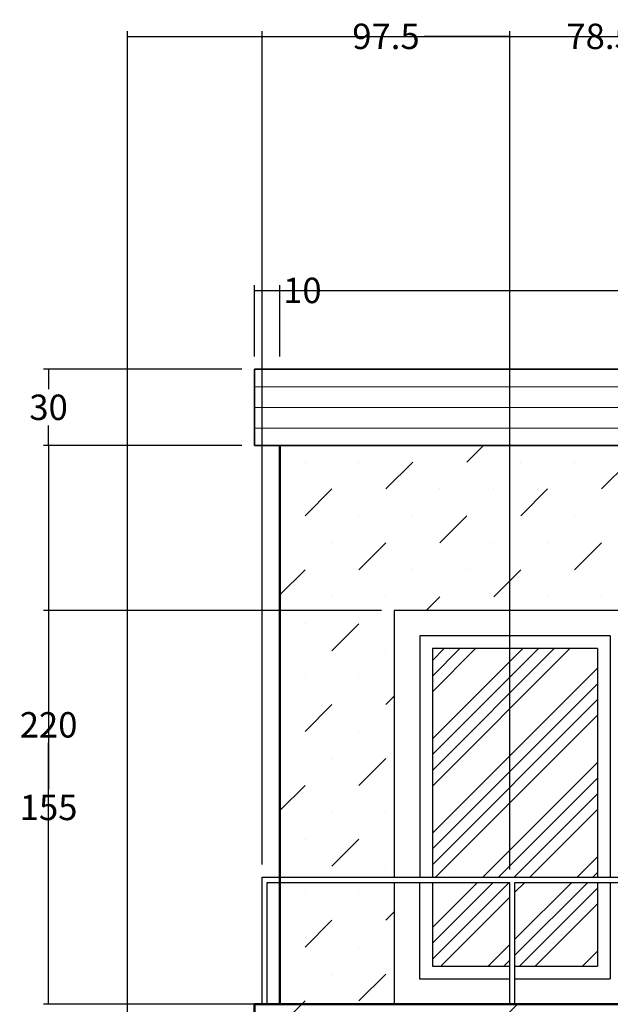
# Model space of a CAD drawing. Units: millimetres. Extents: x 301 to 1039, y -12 to 673.
# Tile 3 of 6: x 301 to 534, y 285 to 673. Entities that reach past the tile are written whole.
import ezdxf

# ---------------------------------------------------------------- set-up
doc = ezdxf.new("R2010")
doc.units = ezdxf.units.MM
doc.header["$MEASUREMENT"] = 0
for name, color, linetype, lineweight in [('A-ANNO-DIMS', 2, 'Continuous', 18), ('A-FLOR-HRAL', 6, 'Continuous', 25), ('A-GLAZ', 4, 'Continuous', 25), ('A-GLAZ-PATT', 8, 'Continuous', 13), ('A-ROOF', 1, 'Continuous', 35), ('A-WALL', 7, 'Continuous', 50), ('A-WALL-PATT', 9, 'Continuous', 13)]:
    doc.layers.add(name, color=color, linetype=linetype, lineweight=lineweight)
doc.styles.get("Standard").update_dxf_attribs({"font": 'arial.ttf'})
doc.dimstyles.get("Standard").update_dxf_attribs({"dimtxt": 10, "dimasz": 0.18, "dimexe": 2, "dimexo": 5, "dimgap": 2, "dimtad": 0, "dimtih": 1, "dimtoh": 1, "dimdec": 0, "dimzin": 0, "dimdsep": 46, "dimtxsty": 'Standard', "dimcen": 0.09, "dimadec": 0, "dimazin": 0, "dimtfac": 1, "dimtdec": 0, "dimtofl": 0, "dimtmove": 0, "dimatfit": 3, "dimfxl": 1, "dimtolj": 1, "dimtzin": 0, "dimarcsym": 0})

# ---------------------------------------------------------------- blocks, each defined once
blk = doc.blocks.new('WIN-SASH-UPPER')
for p, q in [((623.79, 430.09), (548.79, 430.09)), ((548.79, 430.09), (548.79, 400.52)), ((623.79, 430.09), (623.79, 400.52)), ((618.79, 425.09), (553.79, 425.09)), ((553.79, 425.09), (553.79, 400.52)), ((618.79, 425.09), (618.79, 400.52)), ((548.79, 400.52), (548.79, 335.09)), ((553.79, 400.52), (553.79, 335.09)), ((618.79, 400.52), (618.79, 335.09)), ((623.79, 400.52), (623.79, 335.09))]:
    blk.add_line(p, q)
blk = doc.blocks.new('*D20')
at = {"layer": 'A-ANNO-DIMS', "color": 0, "lineweight": -2, "transparency": 16777216}
for p, q in [((343.79, 30.09), (343.79, 668.09)), ((953.79, 30.09), (953.79, 668.09)), ((343.97, 666.09), (635.73, 666.09)), ((953.61, 666.09), (661.85, 666.09))]:
    blk.add_line(p, q, dxfattribs=at)
at = {"layer": 'A-ANNO-DIMS', "color": 0, "transparency": 16777216}
for points in [[(343.97, 666.12), (343.97, 666.06), (343.79, 666.09)], [(953.61, 666.12), (953.61, 666.06), (953.79, 666.09)]]:
    blk.add_solid(points, dxfattribs=at)
at = {"layer": 'Defpoints', "color": 0, "transparency": 16777216}
for p in [(953.79, 666.09), (343.79, 25.09), (953.79, 25.09)]:
    blk.add_point(p, dxfattribs=at)
at = {"layer": 'A-ANNO-DIMS', "color": 0, "transparency": 16777216, "insert": (648.79, 666.09), "char_height": 10, "attachment_point": 5}
blk.add_mtext('\\A1;610', dxfattribs=at)
blk = doc.blocks.new('*D35')
at = {"layer": 'A-ANNO-DIMS', "color": 0, "lineweight": -2, "transparency": 16777216}
for p, q in [((388.79, 505.09), (310.79, 505.09)), ((312.79, 504.91), (312.79, 402.19)), ((312.79, 285.27), (312.79, 387.98)), ((388.79, 285.09), (310.79, 285.09))]:
    blk.add_line(p, q, dxfattribs=at)
at = {"layer": 'A-ANNO-DIMS', "color": 0, "transparency": 16777216}
for points in [[(312.76, 504.91), (312.82, 504.91), (312.79, 505.09)], [(312.76, 285.27), (312.82, 285.27), (312.79, 285.09)]]:
    blk.add_solid(points, dxfattribs=at)
at = {"layer": 'Defpoints', "color": 0, "transparency": 16777216}
for p in [(312.79, 505.09), (393.79, 505.09), (393.79, 285.09)]:
    blk.add_point(p, dxfattribs=at)
at = {"layer": 'A-ANNO-DIMS', "color": 0, "transparency": 16777216, "insert": (312.79, 395.09), "char_height": 10, "attachment_point": 5}
blk.add_mtext('\\A1;220', dxfattribs=at)
blk = doc.blocks.new('*D36')
at = {"layer": 'A-ANNO-DIMS', "color": 0, "lineweight": -2, "transparency": 16777216}
for p, q in [((388.79, 535.09), (310.79, 535.09)), ((312.79, 534.91), (312.79, 527.2)), ((312.79, 505.27), (312.79, 512.98)), ((388.79, 505.09), (310.79, 505.09))]:
    blk.add_line(p, q, dxfattribs=at)
at = {"layer": 'A-ANNO-DIMS', "color": 0, "transparency": 16777216}
for points in [[(312.76, 534.91), (312.82, 534.91), (312.79, 535.09)], [(312.76, 505.27), (312.82, 505.27), (312.79, 505.09)]]:
    blk.add_solid(points, dxfattribs=at)
at = {"layer": 'Defpoints', "color": 0, "transparency": 16777216}
for p in [(312.79, 535.09), (393.79, 535.09), (393.79, 505.09)]:
    blk.add_point(p, dxfattribs=at)
at = {"layer": 'A-ANNO-DIMS', "color": 0, "transparency": 16777216, "insert": (312.79, 520.09), "char_height": 10, "attachment_point": 5}
blk.add_mtext('\\A1;30', dxfattribs=at)
blk = doc.blocks.new('*D43')
at = {"layer": 'A-ANNO-DIMS', "color": 0, "lineweight": -2, "transparency": 16777216}
for p, q in [((393.79, 540.09), (393.79, 568.09)), ((393.97, 566.09), (403.61, 566.09)), ((403.79, 540.09), (403.79, 568.09)), ((403.79, 566.09), (403.97, 566.09))]:
    blk.add_line(p, q, dxfattribs=at)
at = {"layer": 'A-ANNO-DIMS', "color": 0, "transparency": 16777216}
for points in [[(393.97, 566.12), (393.97, 566.06), (393.79, 566.09)], [(403.61, 566.12), (403.61, 566.06), (403.79, 566.09)]]:
    blk.add_solid(points, dxfattribs=at)
at = {"layer": 'Defpoints', "color": 0, "transparency": 16777216}
for p in [(403.79, 566.09), (393.79, 535.09), (403.79, 535.09)]:
    blk.add_point(p, dxfattribs=at)
at = {"layer": 'A-ANNO-DIMS', "color": 0, "transparency": 16777216, "insert": (412.64, 566.09), "char_height": 10, "attachment_point": 5}
blk.add_mtext('\\A1;10', dxfattribs=at)
blk = doc.blocks.new('*D44')
at = {"layer": 'A-ANNO-DIMS', "color": 0, "lineweight": -2, "transparency": 16777216}
for p, q in [((403.79, 540.09), (403.79, 568.09)), ((403.97, 566.09), (540.76, 566.09)), ((703.61, 566.09), (566.82, 566.09)), ((703.79, 540.09), (703.79, 568.09))]:
    blk.add_line(p, q, dxfattribs=at)
at = {"layer": 'A-ANNO-DIMS', "color": 0, "transparency": 16777216}
for points in [[(403.97, 566.12), (403.97, 566.06), (403.79, 566.09)], [(703.61, 566.12), (703.61, 566.06), (703.79, 566.09)]]:
    blk.add_solid(points, dxfattribs=at)
at = {"layer": 'Defpoints', "color": 0, "transparency": 16777216}
for p in [(703.79, 566.09), (403.79, 535.09), (703.79, 535.09)]:
    blk.add_point(p, dxfattribs=at)
at = {"layer": 'A-ANNO-DIMS', "color": 0, "transparency": 16777216, "insert": (553.79, 566.09), "char_height": 10, "attachment_point": 5}
blk.add_mtext('\\A1;300', dxfattribs=at)
blk = doc.blocks.new('*D58')
at = {"layer": 'A-ANNO-DIMS', "color": 0, "lineweight": -2, "transparency": 16777216}
for p, q in [((443.79, 440.09), (310.79, 440.09)), ((312.79, 439.91), (312.79, 369.69)), ((312.79, 285.27), (312.79, 355.48)), ((443.79, 285.09), (310.79, 285.09))]:
    blk.add_line(p, q, dxfattribs=at)
at = {"layer": 'A-ANNO-DIMS', "color": 0, "transparency": 16777216}
for points in [[(312.76, 439.91), (312.82, 439.91), (312.79, 440.09)], [(312.76, 285.27), (312.82, 285.27), (312.79, 285.09)]]:
    blk.add_solid(points, dxfattribs=at)
at = {"layer": 'Defpoints', "color": 0, "transparency": 16777216}
for p in [(312.79, 440.09), (448.79, 440.09), (448.79, 285.09)]:
    blk.add_point(p, dxfattribs=at)
at = {"layer": 'A-ANNO-DIMS', "color": 0, "transparency": 16777216, "insert": (312.79, 362.59), "char_height": 10, "attachment_point": 5}
blk.add_mtext('\\A1;155', dxfattribs=at)
blk = doc.blocks.new('*D59')
at = {"layer": 'A-ANNO-DIMS', "color": 0, "lineweight": -2, "transparency": 16777216}
for p, q in [((396.79, 340.09), (396.79, 668.09)), ((494.29, 338.09), (494.29, 668.09)), ((396.97, 666.09), (430.51, 666.09)), ((494.11, 666.09), (460.56, 666.09))]:
    blk.add_line(p, q, dxfattribs=at)
at = {"layer": 'A-ANNO-DIMS', "color": 0, "transparency": 16777216}
for points in [[(396.97, 666.12), (396.97, 666.06), (396.79, 666.09)], [(494.11, 666.12), (494.11, 666.06), (494.29, 666.09)]]:
    blk.add_solid(points, dxfattribs=at)
at = {"layer": 'Defpoints', "color": 0, "transparency": 16777216}
for p in [(494.29, 666.09), (396.79, 335.09), (494.29, 333.09)]:
    blk.add_point(p, dxfattribs=at)
at = {"layer": 'A-ANNO-DIMS', "color": 0, "transparency": 16777216, "insert": (445.54, 666.09), "char_height": 10, "attachment_point": 5}
blk.add_mtext('\\A1;97.5', dxfattribs=at)
blk = doc.blocks.new('*D60')
at = {"layer": 'A-ANNO-DIMS', "color": 0, "lineweight": -2, "transparency": 16777216}
for p, q in [((494.29, 338.09), (494.29, 668.09)), ((572.8, 338.09), (572.8, 668.09)), ((494.47, 666.09), (515.68, 666.09)), ((572.62, 666.09), (551.41, 666.09))]:
    blk.add_line(p, q, dxfattribs=at)
at = {"layer": 'A-ANNO-DIMS', "color": 0, "transparency": 16777216}
for points in [[(494.47, 666.12), (494.47, 666.06), (494.29, 666.09)], [(572.62, 666.12), (572.62, 666.06), (572.8, 666.09)]]:
    blk.add_solid(points, dxfattribs=at)
at = {"layer": 'Defpoints', "color": 0, "transparency": 16777216}
for p in [(572.8, 666.09), (494.29, 333.09), (572.8, 333.09)]:
    blk.add_point(p, dxfattribs=at)
at = {"layer": 'A-ANNO-DIMS', "color": 0, "transparency": 16777216, "insert": (533.54, 666.09), "char_height": 10, "attachment_point": 5}
blk.add_mtext('\\A1;78.51', dxfattribs=at)

msp = doc.modelspace()

# ---------------------------------------------------------------- hatches: boundary and pattern name
at = {"layer": 'A-GLAZ-PATT'}
h = msp.add_hatch(dxfattribs=at)
h.set_pattern_fill('ANSI34', color=256, scale=35)
h.paths.add_polyline_path([(528.788, 400.52), (528.788, 425.088), (463.788, 425.088), (463.788, 400.52), (463.788, 335.088), (528.788, 335.088)])
h.paths.add_polyline_path([(494.288, 333.088), (463.788, 333.088), (463.788, 300.088), (494.288, 300.088)])
h.paths.add_polyline_path([(528.788, 333.088), (496.288, 333.088), (496.288, 300.088), (528.788, 300.088)])
h.paths.add_polyline_path([(618.788, 400.52), (618.788, 425.088), (553.788, 425.088), (553.788, 400.52), (553.788, 335.088), (618.788, 335.088)])
h.paths.add_polyline_path([(618.788, 333.088), (574.798, 333.088), (574.798, 300.088), (618.788, 300.088)])
h.paths.add_polyline_path([(572.798, 333.088), (553.788, 333.088), (553.788, 300.088), (572.798, 300.088)])
h.paths.add_polyline_path([(501.288, 180.088), (433.788, 180.088), (433.788, 110.088), (501.288, 110.088)])
h.paths.add_polyline_path([(573.788, 180.088), (506.288, 180.088), (506.288, 110.088), (573.788, 110.088)])
h.paths.add_polyline_path([(573.788, 210.088), (506.288, 210.088), (506.288, 185.088), (573.788, 185.088)])
h.paths.add_polyline_path([(501.288, 210.088), (433.788, 210.088), (433.788, 185.088), (501.288, 185.088)])
h.paths.add_polyline_path([(797.687, 412.264), (746.687, 412.264), (746.687, 298.264), (797.687, 298.264)])
h.paths.add_polyline_path([(860.687, 412.264), (809.687, 412.264), (809.687, 298.264), (860.687, 298.264)])
at = {"layer": 'A-WALL-PATT'}
h = msp.add_hatch(dxfattribs=at)
h.set_pattern_fill('ANSI31', color=256, scale=65, angle=135)
h.paths.add_polyline_path([(723.788, 535.088), (703.788, 535.088), (403.788, 535.088), (393.788, 535.088), (393.788, 505.088), (403.788, 505.088), (703.788, 505.088), (723.788, 505.088)])
h = msp.add_hatch(dxfattribs=at)
h.set_pattern_fill('MUDST', color=256, scale=60, angle=45)
edge = h.paths.add_edge_path()
edge.add_line((703.788, 505.088), (403.788, 505.088))
edge.add_line((403.788, 505.088), (403.788, 335.088))
edge.add_line((403.788, 335.088), (448.788, 335.088))
edge.add_line((448.788, 335.088), (448.788, 400.52))
edge.add_line((448.788, 400.52), (448.788, 440.088))
edge.add_line((448.788, 440.088), (633.788, 440.088))
edge.add_line((633.788, 440.088), (633.788, 400.52))
edge.add_line((633.788, 400.52), (633.788, 335.088))
edge.add_line((633.788, 335.088), (673.88, 335.088))
edge.add_spline(control_points=[(673.88, 335.088), (673.929, 335.734), (674.283, 339.462), (675.587, 346.794), (678.602, 339.909), (679.226, 336.718), (679.369, 335.088)], knot_values=[26.7052686, 26.7052686, 26.7052686, 26.7052686, 28.3156814, 35.5227919, 39.6456178, 44.5318346, 44.5318346, 44.5318346, 44.5318346], degree=3, periodic=0)
edge.add_line((679.369, 335.088), (703.788, 335.088))
edge.add_line((703.788, 335.088), (703.788, 505.088))
h.paths.add_polyline_path([(681.292, 397.334, -1), (651.292, 397.334, -1)], flags=16)
h.paths.add_polyline_path([(679.292, 397.334, -1), (653.292, 397.334, -1)], flags=0)
h.paths.add_polyline_path([(448.788, 333.088), (403.788, 333.088), (403.788, 285.088), (448.788, 285.088)])
h.paths.add_polyline_path([(613.788, 260.088), (713.788, 260.088), (713.788, 285.088), (403.788, 285.088), (393.788, 285.088), (393.788, 35.088), (403.788, 35.088), (613.788, 35.088)])
h.paths.add_polyline_path([(578.788, 215.088), (578.788, 105.088), (428.788, 105.088), (428.788, 215.088)], flags=16)
h.paths.add_polyline_path([(501.288, 210.088), (501.288, 185.088), (433.788, 185.088), (433.788, 210.088)], flags=0)
h.paths.add_polyline_path([(501.288, 180.088), (501.288, 110.088), (433.788, 110.088), (433.788, 180.088)], flags=0)
h.paths.add_polyline_path([(506.288, 210.088), (573.788, 210.088), (573.788, 185.088), (506.288, 185.088)], flags=0)
h.paths.add_polyline_path([(506.288, 180.088), (573.788, 180.088), (573.788, 110.088), (506.288, 110.088)], flags=0)
edge = h.paths.add_edge_path()
edge.add_spline(control_points=[(675.148, 309.006), (675.282, 309.92), (671.965, 311.304), (670.019, 313.17), (668.379, 316.485), (667.076, 320.028), (669.149, 324.142), (672.687, 322.877), (673.644, 321.553), (673.786, 321.296)], knot_values=[12.4980994, 12.4980994, 12.4980994, 12.4980994, 15.7345293, 18.1242776, 22.0598536, 26.1694355, 29.2709867, 33.3603853, 34.273637, 34.273637, 34.273637, 34.273637], degree=3, periodic=0)
edge.add_spline(control_points=[(673.786, 321.296), (673.373, 322.666), (672.565, 324.662), (673.805, 325.84), (674.246, 326.099)], knot_values=[12.3304253, 12.3304253, 12.3304253, 12.3304253, 16.1943692, 17.6683934, 17.6683934, 17.6683934, 17.6683934], degree=3, periodic=0)
edge.add_spline(control_points=[(674.246, 326.099), (673.92, 328.298), (673.697, 330.39), (673.774, 333.088)], knot_values=[46.2924512, 46.2924512, 46.2924512, 46.2924512, 53.8278009, 53.8278009, 53.8278009, 53.8278009], degree=3, periodic=0)
edge.add_line((673.774, 333.088), (648.788, 333.088))
edge.add_line((648.788, 333.088), (648.788, 285.088))
edge.add_line((648.788, 285.088), (666.788, 285.088))
edge.add_line((666.788, 285.088), (664.215, 309.96))
edge.add_arc((676.288, 385.148), 76.15, 260.87778, 269.14183)
edge = h.paths.add_edge_path()
edge.add_line((703.788, 333.088), (679.453, 333.088))
edge.add_spline(control_points=[(679.453, 333.088), (679.452, 331.277), (679.21, 329.205), (678.936, 327.067), (678.889, 326.706)], knot_values=[17.8386285, 17.8386285, 17.8386285, 17.8386285, 23.5111371, 24.6594022, 24.6594022, 24.6594022, 24.6594022], degree=3, periodic=0)
edge.add_spline(control_points=[(678.889, 326.706), (678.729, 326.741), (678.565, 326.771), (678.396, 326.794)], knot_values=[21.2892091, 21.2892091, 21.2892091, 21.2892091, 21.7264211, 21.7264211, 21.7264211, 21.7264211], degree=3, periodic=0)
edge.add_spline(control_points=[(678.396, 326.794), (678.233, 326.816), (678.067, 326.832), (677.898, 326.842)], knot_values=[20.8675669, 20.8675669, 20.8675669, 20.8675669, 21.2892091, 21.2892091, 21.2892091, 21.2892091], degree=3, periodic=0)
edge.add_spline(control_points=[(677.898, 326.842), (676.995, 326.898), (676.024, 326.786), (675.195, 326.517)], knot_values=[18.611077, 18.611077, 18.611077, 18.611077, 20.8675669, 20.8675669, 20.8675669, 20.8675669], degree=3, periodic=0)
edge.add_spline(control_points=[(675.195, 326.517), (675.029, 326.464), (674.869, 326.404), (674.716, 326.337)], knot_values=[18.1593829, 18.1593829, 18.1593829, 18.1593829, 18.611077, 18.611077, 18.611077, 18.611077], degree=3, periodic=0)
edge.add_spline(control_points=[(674.716, 326.337), (674.55, 326.265), (674.392, 326.186), (674.246, 326.099)], knot_values=[17.6683934, 17.6683934, 17.6683934, 17.6683934, 18.1593829, 18.1593829, 18.1593829, 18.1593829], degree=3, periodic=0)
edge.add_spline(control_points=[(674.246, 326.099), (673.805, 325.84), (672.565, 324.662), (673.373, 322.666), (673.786, 321.296)], knot_values=[12.3304253, 12.3304253, 12.3304253, 12.3304253, 13.8044495, 17.6683934, 17.6683934, 17.6683934, 17.6683934], degree=3, periodic=0)
edge.add_spline(control_points=[(673.786, 321.296), (674.162, 320.613), (674.301, 319.823), (674.341, 318.987)], knot_values=[10.0649388, 10.0649388, 10.0649388, 10.0649388, 12.4980994, 12.4980994, 12.4980994, 12.4980994], degree=3, periodic=0)
edge.add_spline(control_points=[(674.341, 318.987), (674.206, 319.737), (674.024, 320.504), (673.786, 321.296)], knot_values=[10.094462, 10.094462, 10.094462, 10.094462, 12.3304253, 12.3304253, 12.3304253, 12.3304253], degree=3, periodic=0)
edge.add_spline(control_points=[(673.786, 321.296), (673.644, 321.553), (672.687, 322.877), (669.149, 324.142), (667.076, 320.028), (668.379, 316.485), (670.019, 313.17), (671.965, 311.304), (675.282, 309.92), (675.148, 309.006)], knot_values=[12.4980994, 12.4980994, 12.4980994, 12.4980994, 13.4113511, 17.5007497, 20.6023009, 24.7118828, 28.6474588, 31.0372071, 34.273637, 34.273637, 34.273637, 34.273637], degree=3, periodic=0)
edge.add_arc((676.288, 385.148), 76.15, 260.87778, 269.14183, ccw=False)
edge.add_line((664.215, 309.96), (666.788, 285.088))
edge.add_line((666.788, 285.088), (703.788, 285.088))
edge.add_line((703.788, 285.088), (703.788, 333.088))
h.paths.add_polyline_path([(687.234, 308.777), (684.887, 286.088), (667.69, 286.088), (665.343, 308.777, 0.0712952)], flags=16)
h.paths.add_polyline_path([(903.788, 265.672), (713.788, 265.672), (713.788, 260.088), (703.788, 260.088), (703.788, 35.088), (728.788, 35.088), (728.788, 160.088), (878.788, 160.088), (878.788, 35.088), (903.788, 35.088)])

# ---------------------------------------------------------------- linework, layer by layer
at = {"layer": 'A-FLOR-HRAL'}
for p, q in [((396.788, 285.088), (396.788, 335.088)), ((396.788, 335.088), (713.788, 335.088)), ((398.788, 285.088), (398.788, 333.088)), ((398.788, 333.088), (494.288, 333.088)), ((494.288, 285.088), (494.288, 333.088)), ((496.288, 285.088), (496.288, 333.088)), ((496.288, 333.088), (572.798, 333.088)), ((393.788, 285.088), (396.788, 285.088))]:
    msp.add_line(p, q, dxfattribs=at)
at = {"layer": 'A-GLAZ'}
for p, q in [((448.788, 440.088), (448.788, 400.52)), ((633.788, 440.088), (448.788, 440.088)), ((448.788, 400.52), (448.788, 335.088)), ((448.788, 333.088), (448.788, 285.088)), ((458.788, 333.088), (458.788, 295.088)), ((463.788, 333.088), (463.788, 300.088)), ((528.788, 333.088), (528.788, 300.088)), ((533.788, 333.088), (533.788, 295.088)), ((463.788, 300.088), (494.288, 300.088)), ((496.288, 300.088), (528.788, 300.088)), ((458.788, 295.088), (494.288, 295.088)), ((496.288, 295.088), (533.788, 295.088))]:
    msp.add_line(p, q, dxfattribs=at)
at = {"layer": 'A-ROOF'}
for p, q in [((403.788, 535.088), (393.788, 535.088)), ((393.788, 535.088), (393.788, 505.088)), ((703.788, 535.088), (403.788, 535.088)), ((393.788, 505.088), (403.788, 505.088)), ((703.788, 505.088), (403.788, 505.088))]:
    msp.add_line(p, q, dxfattribs=at)
at = {"layer": 'A-WALL'}
for p, q in [((403.788, 505.088), (403.788, 285.088)), ((403.788, 285.088), (393.788, 285.088)), ((393.788, 285.088), (393.788, 35.088)), ((403.788, 285.088), (713.788, 285.088))]:
    msp.add_line(p, q, dxfattribs=at)

# ---------------------------------------------------------------- block references
at = {"layer": 'A-GLAZ'}
msp.add_blockref('WIN-SASH-UPPER', (-90, 0), dxfattribs=at)

# ---------------------------------------------------------------- dimensions: what is measured, and where the dimension line sits
at = {"layer": 'A-ANNO-DIMS'}
for base, p1, p2, override, picture, middle in [((953.788, 666.088), (343.788, 25.088), (953.788, 25.088), {"dimdec": 0, "dimlfac": 1, "dimrnd": 0, "dimzin": 0, "dimdsep": 46, "dimlunit": 2}, '*D20', (648.788, 666.088)), ((494.288, 666.088), (396.788, 335.088), (494.288, 333.088), {"dimdec": 1, "dimlfac": 1, "dimrnd": 0, "dimzin": 0, "dimdsep": 46, "dimlunit": 2}, '*D59', (445.538, 666.088)), ((572.798, 666.088), (494.288, 333.088), (572.798, 333.088), {"dimdec": 2, "dimlfac": 1, "dimrnd": 0, "dimzin": 0, "dimdsep": 46, "dimlunit": 2}, '*D60', (533.543, 666.088)), ((403.788, 566.088), (393.788, 535.088), (403.788, 535.088), {"dimdec": 0, "dimlfac": 1, "dimrnd": 0, "dimzin": 0, "dimdsep": 46, "dimlunit": 2}, '*D43', (412.643, 566.088)), ((703.788, 566.088), (403.788, 535.088), (703.788, 535.088), {"dimdec": 0, "dimlfac": 1, "dimrnd": 0, "dimzin": 0, "dimdsep": 46, "dimlunit": 2}, '*D44', (553.788, 566.088))]:
    dim = msp.add_linear_dim(base=base, p1=p1, p2=p2, dimstyle='Standard', override=override, dxfattribs=at)
    dim.commit()
    dim.dimension.update_dxf_attribs({"geometry": picture, "text_midpoint": middle})
for base, p1, p2, picture, middle in [((312.788, 535.088), (393.788, 505.088), (393.788, 535.088), '*D36', (312.788, 520.088)), ((312.788, 505.088), (393.788, 285.088), (393.788, 505.088), '*D35', (312.788, 395.088)), ((312.788, 440.088), (448.788, 285.088), (448.788, 440.088), '*D58', (312.788, 362.588))]:
    dim = msp.add_linear_dim(base=base, p1=p1, p2=p2, angle=90, dimstyle='Standard', override={"dimdec": 0, "dimlfac": 1, "dimrnd": 0, "dimzin": 0, "dimdsep": 46, "dimlunit": 2}, dxfattribs=at)
    dim.commit()
    dim.dimension.update_dxf_attribs({"geometry": picture, "text_midpoint": middle})

doc.saveas('drawing.dxf')
